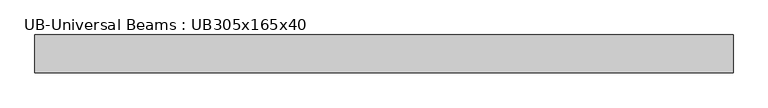
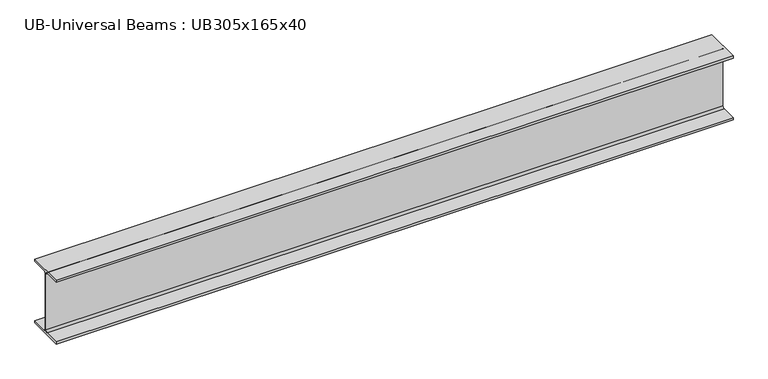
"""IFC4 building model written with IfcOpenShell, lengths in millimetres: beam geometry, UB-Universal Beams : UB305x165x40."""

from ifc_helpers import new_model, si_unit, point, frame, frame_2d, origin, place, context, project, spatial, polyline, circle_curve, trimmed, segment, composite_curve, outline, extrude, source, transform, mapped, element, save


def ub_universal_beams_ub305x165x40_59f247e4(model_context):
    return source(origin(), model_context, "Body", "SweptSolid", [
        extrude(outline(composite_curve([segment(polyline([(82.5, -141.5), (82.5, -151.7), (-82.5, -151.7), (-82.5, -141.5), (-11.9, -141.5)]), True, "CONTINUOUS"), segment(trimmed(circle_curve(frame_2d((-11.9, -132.6)), 8.9), [point((-11.9, -141.5))], [point((-3.0, -132.6))], True, "CARTESIAN"), True, "CONTINUOUS"), segment(polyline([(-3.0, -132.6), (-3.0, 132.6)]), True, "CONTINUOUS"), segment(trimmed(circle_curve(frame_2d((-11.9, 132.6)), 8.9), [point((-3.0, 132.6))], [point((-11.9, 141.5))], True, "CARTESIAN"), True, "CONTINUOUS"), segment(polyline([(-11.9, 141.5), (-82.5, 141.5), (-82.5, 151.7), (82.5, 151.7), (82.5, 141.5), (11.9, 141.5)]), True, "CONTINUOUS"), segment(trimmed(circle_curve(frame_2d((11.9, 132.6)), 8.9), [point((11.9, 141.5))], [point((3.0, 132.6))], True, "CARTESIAN"), True, "CONTINUOUS"), segment(polyline([(3.0, 132.6), (3.0, -132.6)]), True, "CONTINUOUS"), segment(trimmed(circle_curve(frame_2d((11.9, -132.6)), 8.9), [point((3.0, -132.6))], [point((11.9, -141.5))], True, "CARTESIAN"), True, "CONTINUOUS"), segment(polyline([(11.9, -141.5), (82.5, -141.5)]), True, "CONTINUOUS")], self_intersect=False)), frame((-1617.85, 0.0, 0.0), z_axis=(1.0, 0.0, 0.0), x_axis=(0.0, 1.0, 0.0)), (0.0, 0.0, 1.0), 3040.5),
    ])


if __name__ == "__main__":
    model = new_model("IFC4")
    model_context = context("Model", 3, world=origin())
    ifc_project = project(units=[si_unit("LENGTHUNIT", "METRE", prefix="MILLI")], contexts=[model_context])
    site = spatial("IfcSite", under=ifc_project)
    building = spatial("IfcBuilding", under=site)
    placement = place(None, origin())
    ub_universal_beams_ub305x165x40_shape = ub_universal_beams_ub305x165x40_59f247e4(model_context)
    element("IfcBeam", 1, ObjectType="UB-Universal Beams : UB305x165x40", at=placement, inside=building, context=model_context, shape_type="MappedRepresentation", body=[
        mapped(ub_universal_beams_ub305x165x40_shape, transform((0.0, 0.0, 0.0), x_axis=(1.0, 0.0, 0.0), y_axis=(0.0, 1.0, 0.0), z_axis=(0.0, 0.0, 1.0))),
    ])
    save(model, "model.ifc")

# Revit data of these elements
# Type "UB-Universal Beams : UB305x165x40"
#   Section Name Key = "UB305X165X40"
#   Width = 16.5 cm
#   Web Thickness = 0.6 cm
#   Web Fillet = 0.89 cm
#   Warping Constant = 164000.0 cm⁶
#   Torsional Moment of Inertia = 14.70 cm⁴
#   Section Area = 51.3 cm²
#   Plastic Modulus weak axis = 142.0 cm³
#   Plastic Modulus strong axis = 623.0 cm³
#   Nominal Weight = 40.2999 kgf/m
#   Moment of Inertia weak axis = 764.00 cm⁴
#   Moment of Inertia strong axis = 8503.00 cm⁴
#   Height = 30.34 cm
#   Flange Thickness = 1.02 cm
#   Elastic Modulus weak axis = 92.6 cm³
#   Elastic Modulus strong axis = 560.0 cm³
#   Centroid Vertical = 15.17 cm
#   Centroid Horizontal = 8.25 cm
#   Bolt Spacing = 9.0 cm
#   Length [instance default] = 1.5 m
#   Structural Material [instance default] = Metal - Steel 43-275
#   Type Comments = ""
#   Assembly Code = ""
# Element 1 (IfcBeam, "UB-Universal Beams : UB305x165x40")
#   Materials on its faces: "Metal - Steel 43-275"
# Materials
#   "Metal - Steel 43-275": class "Metal", colour RGB 247 247 247, transparency 0, Cost = 0
